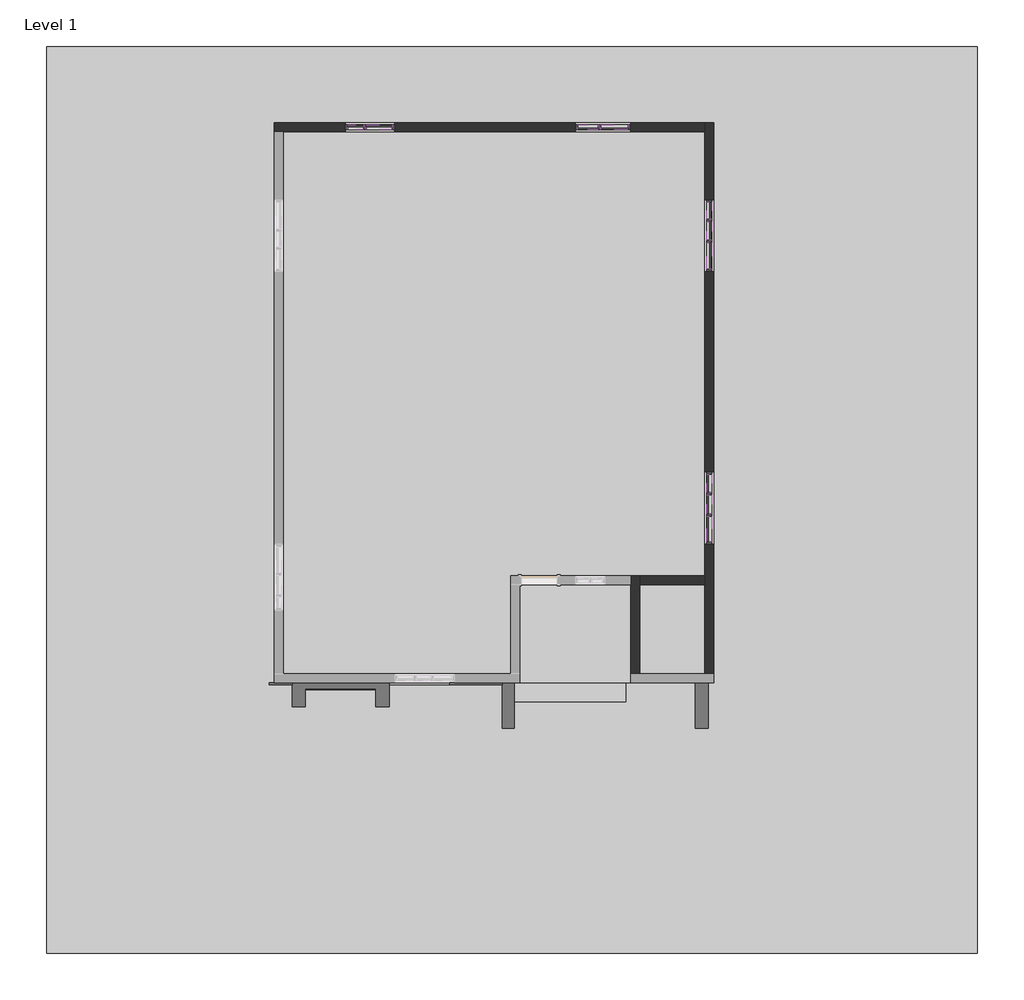
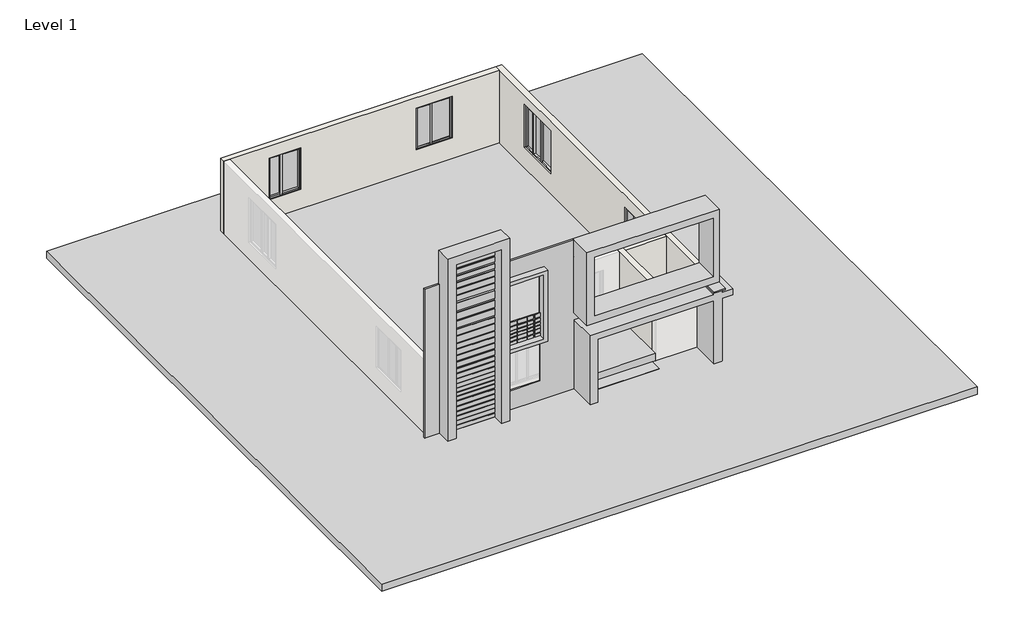
# One storey, part 2 of 2: 34 members, 10 plates, 4 walls, 2 proxies.
"""IFC4 building model written with IfcOpenShell, lengths in millimetres."""

from ifc_helpers import new_model, si_unit, origin, origin_with_axes, place, context, project, spatial, polyline, outline, extrude, faceted_brep, transform, mapped, element, save
from components import generic_models_1_generic_models_1_010c0d49, generic_models_2_generic_models_2_25274e54, member_dc106669, member_969ca954, member_86d06fe4, member_dad99500, member_5e920210, member_530c9cc4, member_2b79973d, member_c33c434a, member_337b6441, member_f67b4128, member_6fb4a552, member_0b7646a3, member_b956c4f6, member_d8304dce, member_273748f4, member_7c181f63, member_bc773a83, member_183d059d, system_panel_glazed_46d50955, system_panel_glazed_6f1fa804, system_panel_glazed_7e68e824, system_panel_glazed_aca50f87, system_panel_glazed_bef0ddaa, system_panel_glazed_29222c04, system_panel_glazed_73ac8250, system_panel_glazed_52b4f5c1, system_panel_glazed_3b3b315d, system_panel_glazed_762caeb2

model = new_model("IFC4")

# Units and contexts
model_context = context("Model", 3, world=origin())
ifc_project = project(units=[si_unit("LENGTHUNIT", "METRE", prefix="MILLI")], contexts=[model_context])

# Site, building, storey
site = spatial("IfcSite", under=ifc_project)
building = spatial("IfcBuilding", under=site)
storey = spatial("IfcBuildingStorey", under=building, Name="Level 1", Elevation=0.0)

# Proxies
placement = place(None, origin())
generic_models_1_generic_models_1_shape = generic_models_1_generic_models_1_010c0d49(model_context)
element("IfcBuildingElementProxy", 1, Name="Generic Models 1 : Generic Models 1", ObjectType="Generic Models 1 : Generic Models 1", at=placement, inside=storey, context=model_context, shape_type="MappedRepresentation", body=[
    mapped(generic_models_1_generic_models_1_shape, transform((0.0, 0.0, 0.0), x_axis=(1.0, 0.0, 0.0), y_axis=(0.0, 1.0, 0.0), z_axis=(0.0, 0.0, 1.0))),
])
generic_models_2_generic_models_2_shape = generic_models_2_generic_models_2_25274e54(model_context)
element("IfcBuildingElementProxy", 2, Name="Generic Models 2 : Generic Models 2", ObjectType="Generic Models 2 : Generic Models 2", at=placement, inside=storey, context=model_context, shape_type="MappedRepresentation", body=[
    mapped(generic_models_2_generic_models_2_shape, transform((-134.3868469, 0.0, -162.5364257), x_axis=(1.0, 0.0, 0.0), y_axis=(0.0, 1.0, 0.0), z_axis=(0.0, 0.0, 1.0))),
])

# Members
member_shape = member_dc106669(model_context)
element("IfcMember", 3, ObjectType="Rectangular Mullion : 2.5\" x 5\" rectangular", at=placement, inside=storey, context=model_context, shape_type="MappedRepresentation", body=[
    mapped(member_shape, transform((-14463.3781629, -790.0678064, 2550.7938638), x_axis=(0.0, 0.0, 1.0), y_axis=(0.0, -1.0, 0.0), z_axis=(1.0, 0.0, 0.0))),
])
element("IfcMember", 4, ObjectType="Rectangular Mullion : 2.5\" x 5\" rectangular", at=placement, inside=storey, context=model_context, shape_type="MappedRepresentation", body=[
    mapped(member_shape, transform((-14876.1281629, -790.0678064, 803.2813363), x_axis=(0.0, 0.0, -1.0), y_axis=(0.0, -1.0, 0.0), z_axis=(-1.0, 0.0, 0.0))),
])
member_2_shape = member_969ca954(model_context)
element("IfcMember", 5, ObjectType="Rectangular Mullion : 2.5\" x 5\" rectangular", at=placement, inside=storey, context=model_context, shape_type="MappedRepresentation", body=[
    mapped(member_2_shape, transform((-5719.4281629, -10029.3178064, 840.8595188), x_axis=(0.0, 0.0, -1.0), y_axis=(1.0, 0.0, 0.0), z_axis=(0.0, -1.0, 0.0))),
])
member_3_shape = member_86d06fe4(model_context)
element("IfcMember", 6, ObjectType="Rectangular Mullion : 2.5\" x 5\" rectangular", at=placement, inside=storey, context=model_context, shape_type="MappedRepresentation", body=[
    mapped(member_3_shape, transform((-5719.4281629, -10575.4178064, 840.8595188), x_axis=(0.0, 0.0, -1.0), y_axis=(1.0, 0.0, 0.0), z_axis=(0.0, -1.0, 0.0))),
])
member_4_shape = member_dad99500(model_context)
element("IfcMember", 7, ObjectType="Rectangular Mullion : 2.5\" x 5\" rectangular", at=placement, inside=storey, context=model_context, shape_type="MappedRepresentation", body=[
    mapped(member_4_shape, transform((-5719.4281629, -11280.2678064, 840.8595188), x_axis=(0.0, 0.0, -1.0), y_axis=(1.0, 0.0, 0.0), z_axis=(0.0, -1.0, 0.0))),
])
member_5_shape = member_5e920210(model_context)
element("IfcMember", 8, ObjectType="Rectangular Mullion : 2.5\" x 5\" rectangular", at=placement, inside=storey, context=model_context, shape_type="MappedRepresentation", body=[
    mapped(member_5_shape, transform((-5719.4281629, -10607.1678064, 840.8595188), x_axis=(0.0, 1.0, 0.0), y_axis=(1.0, 0.0, 0.0), z_axis=(0.0, 0.0, -1.0))),
])
element("IfcMember", 9, ObjectType="Rectangular Mullion : 2.5\" x 5\" rectangular", at=placement, inside=storey, context=model_context, shape_type="MappedRepresentation", body=[
    mapped(member_5_shape, transform((-5719.4281629, -10061.0678064, 840.8595188), x_axis=(0.0, 1.0, 0.0), y_axis=(1.0, 0.0, 0.0), z_axis=(0.0, 0.0, -1.0))),
])
element("IfcMember", 10, ObjectType="Rectangular Mullion : 2.5\" x 5\" rectangular", at=placement, inside=storey, context=model_context, shape_type="MappedRepresentation", body=[
    mapped(member_3_shape, transform((-5719.4281629, -10092.8178064, 2522.9339832), x_axis=(0.0, 0.0, 1.0), y_axis=(1.0, 0.0, 0.0), z_axis=(0.0, 1.0, 0.0))),
])
element("IfcMember", 11, ObjectType="Rectangular Mullion : 2.5\" x 5\" rectangular", at=placement, inside=storey, context=model_context, shape_type="MappedRepresentation", body=[
    mapped(member_4_shape, transform((-5719.4281629, -10638.9178064, 2522.9339832), x_axis=(0.0, 0.0, 1.0), y_axis=(1.0, 0.0, 0.0), z_axis=(0.0, 1.0, 0.0))),
])
element("IfcMember", 12, ObjectType="Rectangular Mullion : 2.5\" x 5\" rectangular", at=placement, inside=storey, context=model_context, shape_type="MappedRepresentation", body=[
    mapped(member_2_shape, transform((-5719.4281629, -9578.4678064, 2522.9339832), x_axis=(0.0, 0.0, 1.0), y_axis=(1.0, 0.0, 0.0), z_axis=(0.0, 1.0, 0.0))),
])
member_6_shape = member_530c9cc4(model_context)
element("IfcMember", 13, ObjectType="Rectangular Mullion : 2.5\" x 5\" rectangular", at=placement, inside=storey, context=model_context, shape_type="MappedRepresentation", body=[
    mapped(member_6_shape, transform((-5719.4281629, -9514.9678064, 840.8595188), x_axis=(0.0, 1.0, 0.0), y_axis=(1.0, 0.0, 0.0), z_axis=(0.0, 0.0, -1.0))),
])
element("IfcMember", 14, ObjectType="Rectangular Mullion : 2.5\" x 5\" rectangular", at=placement, inside=storey, context=model_context, shape_type="MappedRepresentation", body=[
    mapped(member_6_shape, transform((-5719.4281629, -11343.7678064, 2522.9339832), x_axis=(0.0, -1.0, 0.0), y_axis=(1.0, 0.0, 0.0), z_axis=(0.0, 0.0, 1.0))),
])
member_7_shape = member_2b79973d(model_context)
element("IfcMember", 15, ObjectType="Rectangular Mullion : 2.5\" x 5\" rectangular", at=placement, inside=storey, context=model_context, shape_type="MappedRepresentation", body=[
    mapped(member_7_shape, transform((-5719.4281629, -3653.9178064, 2661.4285089), x_axis=(0.0, 0.0, 1.0), y_axis=(-1.0, 0.0, 0.0), z_axis=(0.0, -1.0, 0.0))),
])
member_8_shape = member_c33c434a(model_context)
element("IfcMember", 16, ObjectType="Rectangular Mullion : 2.5\" x 5\" rectangular", at=placement, inside=storey, context=model_context, shape_type="MappedRepresentation", body=[
    mapped(member_8_shape, transform((-5719.4281629, -4384.1678064, 2661.4285089), x_axis=(0.0, 0.0, 1.0), y_axis=(-1.0, 0.0, 0.0), z_axis=(0.0, -1.0, 0.0))),
])
member_9_shape = member_337b6441(model_context)
element("IfcMember", 17, ObjectType="Rectangular Mullion : 2.5\" x 5\" rectangular", at=placement, inside=storey, context=model_context, shape_type="MappedRepresentation", body=[
    mapped(member_9_shape, transform((-5719.4281629, -3152.2678064, 856.0019171), x_axis=(0.0, -1.0, 0.0), y_axis=(-1.0, 0.0, 0.0), z_axis=(0.0, 0.0, -1.0))),
])
element("IfcMember", 18, ObjectType="Rectangular Mullion : 2.5\" x 5\" rectangular", at=placement, inside=storey, context=model_context, shape_type="MappedRepresentation", body=[
    mapped(member_9_shape, transform((-5719.4281629, -3685.6678064, 856.0019171), x_axis=(0.0, -1.0, 0.0), y_axis=(-1.0, 0.0, 0.0), z_axis=(0.0, 0.0, -1.0))),
])
element("IfcMember", 19, ObjectType="Rectangular Mullion : 2.5\" x 5\" rectangular", at=placement, inside=storey, context=model_context, shape_type="MappedRepresentation", body=[
    mapped(member_7_shape, transform((-5719.4281629, -3184.0178064, 856.0019171), x_axis=(0.0, 0.0, -1.0), y_axis=(-1.0, 0.0, 0.0), z_axis=(0.0, 1.0, 0.0))),
])
element("IfcMember", 20, ObjectType="Rectangular Mullion : 2.5\" x 5\" rectangular", at=placement, inside=storey, context=model_context, shape_type="MappedRepresentation", body=[
    mapped(member_8_shape, transform((-5719.4281629, -3717.4178064, 856.0019171), x_axis=(0.0, 0.0, -1.0), y_axis=(-1.0, 0.0, 0.0), z_axis=(0.0, 1.0, 0.0))),
])
member_10_shape = member_f67b4128(model_context)
element("IfcMember", 21, ObjectType="Rectangular Mullion : 2.5\" x 5\" rectangular", at=placement, inside=storey, context=model_context, shape_type="MappedRepresentation", body=[
    mapped(member_10_shape, transform((-5719.4281629, -4447.6678064, 856.0019171), x_axis=(0.0, -1.0, 0.0), y_axis=(-1.0, 0.0, 0.0), z_axis=(0.0, 0.0, -1.0))),
])
member_11_shape = member_6fb4a552(model_context)
element("IfcMember", 22, ObjectType="Rectangular Mullion : 2.5\" x 5\" rectangular", at=placement, inside=storey, context=model_context, shape_type="MappedRepresentation", body=[
    mapped(member_11_shape, transform((-5719.4281629, -3120.5178064, 2661.4285089), x_axis=(0.0, 0.0, 1.0), y_axis=(-1.0, 0.0, 0.0), z_axis=(0.0, -1.0, 0.0))),
])
element("IfcMember", 23, ObjectType="Rectangular Mullion : 2.5\" x 5\" rectangular", at=placement, inside=storey, context=model_context, shape_type="MappedRepresentation", body=[
    mapped(member_11_shape, transform((-5719.4281629, -2682.3678064, 856.0019171), x_axis=(0.0, 0.0, -1.0), y_axis=(-1.0, 0.0, 0.0), z_axis=(0.0, 1.0, 0.0))),
])
element("IfcMember", 24, ObjectType="Rectangular Mullion : 2.5\" x 5\" rectangular", at=placement, inside=storey, context=model_context, shape_type="MappedRepresentation", body=[
    mapped(member_10_shape, transform((-5719.4281629, -2618.8678064, 2661.4285089), x_axis=(0.0, 1.0, 0.0), y_axis=(-1.0, 0.0, 0.0), z_axis=(0.0, 0.0, 1.0))),
])
member_12_shape = member_0b7646a3(model_context)
element("IfcMember", 25, ObjectType="Rectangular Mullion : 2.5\" x 5\" rectangular", at=placement, inside=storey, context=model_context, shape_type="MappedRepresentation", body=[
    mapped(member_12_shape, transform((-9046.8281629, -790.0678064, 2606.6947773), x_axis=(0.0, 0.0, 1.0), y_axis=(0.0, 1.0, 0.0), z_axis=(-1.0, 0.0, 0.0))),
])
member_13_shape = member_b956c4f6(model_context)
element("IfcMember", 26, ObjectType="Rectangular Mullion : 2.5\" x 5\" rectangular", at=placement, inside=storey, context=model_context, shape_type="MappedRepresentation", body=[
    mapped(member_13_shape, transform((-8468.9781629, -790.0678064, 2606.6947773), x_axis=(0.0, 0.0, 1.0), y_axis=(0.0, 1.0, 0.0), z_axis=(-1.0, 0.0, 0.0))),
])
member_14_shape = member_d8304dce(model_context)
element("IfcMember", 27, ObjectType="Rectangular Mullion : 2.5\" x 5\" rectangular", at=placement, inside=storey, context=model_context, shape_type="MappedRepresentation", body=[
    mapped(member_14_shape, transform((-8500.7281629, -790.0678064, 862.6148637), x_axis=(-1.0, 0.0, 0.0), y_axis=(0.0, 1.0, 0.0), z_axis=(0.0, 0.0, -1.0))),
])
element("IfcMember", 28, ObjectType="Rectangular Mullion : 2.5\" x 5\" rectangular", at=placement, inside=storey, context=model_context, shape_type="MappedRepresentation", body=[
    mapped(member_12_shape, transform((-8532.4781629, -790.0678064, 862.6148637), x_axis=(0.0, 0.0, -1.0), y_axis=(0.0, 1.0, 0.0), z_axis=(1.0, 0.0, 0.0))),
])
element("IfcMember", 29, ObjectType="Rectangular Mullion : 2.5\" x 5\" rectangular", at=placement, inside=storey, context=model_context, shape_type="MappedRepresentation", body=[
    mapped(member_13_shape, transform((-7764.1281629, -790.0678064, 862.6148637), x_axis=(0.0, 0.0, -1.0), y_axis=(0.0, 1.0, 0.0), z_axis=(1.0, 0.0, 0.0))),
])
member_15_shape = member_273748f4(model_context)
element("IfcMember", 30, ObjectType="Rectangular Mullion : 2.5\" x 5\" rectangular", at=placement, inside=storey, context=model_context, shape_type="MappedRepresentation", body=[
    mapped(member_15_shape, transform((-9110.3281629, -790.0678064, 862.6148637), x_axis=(-1.0, 0.0, 0.0), y_axis=(0.0, 1.0, 0.0), z_axis=(0.0, 0.0, -1.0))),
])
element("IfcMember", 31, ObjectType="Rectangular Mullion : 2.5\" x 5\" rectangular", at=placement, inside=storey, context=model_context, shape_type="MappedRepresentation", body=[
    mapped(member_15_shape, transform((-7700.6281629, -790.0678064, 2606.6947773), x_axis=(1.0, 0.0, 0.0), y_axis=(0.0, 1.0, 0.0), z_axis=(0.0, 0.0, 1.0))),
])
member_16_shape = member_7c181f63(model_context)
element("IfcMember", 32, ObjectType="Rectangular Mullion : 2.5\" x 5\" rectangular", at=placement, inside=storey, context=model_context, shape_type="MappedRepresentation", body=[
    mapped(member_16_shape, transform((-13745.8281629, -790.0678064, 2550.7938638), x_axis=(0.0, 0.0, 1.0), y_axis=(0.0, -1.0, 0.0), z_axis=(1.0, 0.0, 0.0))),
])
member_17_shape = member_bc773a83(model_context)
element("IfcMember", 33, ObjectType="Rectangular Mullion : 2.5\" x 5\" rectangular", at=placement, inside=storey, context=model_context, shape_type="MappedRepresentation", body=[
    mapped(member_17_shape, transform((-14431.6281629, -790.0678064, 803.2813363), x_axis=(1.0, 0.0, 0.0), y_axis=(0.0, -1.0, 0.0), z_axis=(0.0, 0.0, -1.0))),
])
element("IfcMember", 34, ObjectType="Rectangular Mullion : 2.5\" x 5\" rectangular", at=placement, inside=storey, context=model_context, shape_type="MappedRepresentation", body=[
    mapped(member_16_shape, transform((-14399.8781629, -790.0678064, 803.2813363), x_axis=(0.0, 0.0, -1.0), y_axis=(0.0, -1.0, 0.0), z_axis=(-1.0, 0.0, 0.0))),
])
member_18_shape = member_183d059d(model_context)
element("IfcMember", 35, ObjectType="Rectangular Mullion : 2.5\" x 5\" rectangular", at=placement, inside=storey, context=model_context, shape_type="MappedRepresentation", body=[
    mapped(member_18_shape, transform((-14939.6281629, -790.0678064, 2550.7938638), x_axis=(-1.0, 0.0, 0.0), y_axis=(0.0, -1.0, 0.0), z_axis=(0.0, 0.0, 1.0))),
])
element("IfcMember", 36, ObjectType="Rectangular Mullion : 2.5\" x 5\" rectangular", at=placement, inside=storey, context=model_context, shape_type="MappedRepresentation", body=[
    mapped(member_18_shape, transform((-13682.3281629, -790.0678064, 803.2813363), x_axis=(1.0, 0.0, 0.0), y_axis=(0.0, -1.0, 0.0), z_axis=(0.0, 0.0, -1.0))),
])

# Plates
system_panel_glazed_shape = system_panel_glazed_46d50955(model_context)
element("IfcPlate", 37, ObjectType="System Panel : Glazed", at=placement, inside=storey, context=model_context, shape_type="MappedRepresentation", body=[
    mapped(system_panel_glazed_shape, transform((-5719.4281629, -10959.5928064, 904.3595188), x_axis=(0.0, 1.0, 0.0), y_axis=(-1.0, 0.0, 0.0), z_axis=(0.0, 0.0, 1.0))),
])
system_panel_glazed_2_shape = system_panel_glazed_6f1fa804(model_context)
element("IfcPlate", 38, ObjectType="System Panel : Glazed", at=placement, inside=storey, context=model_context, shape_type="MappedRepresentation", body=[
    mapped(system_panel_glazed_2_shape, transform((-5719.4281629, -10334.1178064, 904.3595188), x_axis=(0.0, 1.0, 0.0), y_axis=(-1.0, 0.0, 0.0), z_axis=(0.0, 0.0, 1.0))),
])
system_panel_glazed_3_shape = system_panel_glazed_7e68e824(model_context)
element("IfcPlate", 39, ObjectType="System Panel : Glazed", at=placement, inside=storey, context=model_context, shape_type="MappedRepresentation", body=[
    mapped(system_panel_glazed_3_shape, transform((-5719.4281629, -9803.8928064, 904.3595188), x_axis=(0.0, 1.0, 0.0), y_axis=(-1.0, 0.0, 0.0), z_axis=(0.0, 0.0, 1.0))),
])
system_panel_glazed_4_shape = system_panel_glazed_aca50f87(model_context)
element("IfcPlate", 40, ObjectType="System Panel : Glazed", at=placement, inside=storey, context=model_context, shape_type="MappedRepresentation", body=[
    mapped(system_panel_glazed_4_shape, transform((-5719.4281629, -4050.7928064, 919.5019171), x_axis=(0.0, -1.0, 0.0), y_axis=(1.0, 0.0, 0.0), z_axis=(0.0, 0.0, 1.0))),
])
system_panel_glazed_5_shape = system_panel_glazed_bef0ddaa(model_context)
element("IfcPlate", 41, ObjectType="System Panel : Glazed", at=placement, inside=storey, context=model_context, shape_type="MappedRepresentation", body=[
    mapped(system_panel_glazed_5_shape, transform((-5719.4281629, -3418.9678064, 919.5019171), x_axis=(0.0, -1.0, 0.0), y_axis=(1.0, 0.0, 0.0), z_axis=(0.0, 0.0, 1.0))),
])
system_panel_glazed_6_shape = system_panel_glazed_29222c04(model_context)
element("IfcPlate", 42, ObjectType="System Panel : Glazed", at=placement, inside=storey, context=model_context, shape_type="MappedRepresentation", body=[
    mapped(system_panel_glazed_6_shape, transform((-5719.4281629, -2901.4428064, 919.5019171), x_axis=(0.0, -1.0, 0.0), y_axis=(1.0, 0.0, 0.0), z_axis=(0.0, 0.0, 1.0))),
])
system_panel_glazed_7_shape = system_panel_glazed_73ac8250(model_context)
element("IfcPlate", 43, ObjectType="System Panel : Glazed", at=placement, inside=storey, context=model_context, shape_type="MappedRepresentation", body=[
    mapped(system_panel_glazed_7_shape, transform((-8116.5531629, -790.0678064, 926.1148637), x_axis=(-1.0, 0.0, 0.0), y_axis=(0.0, -1.0, 0.0), z_axis=(0.0, 0.0, 1.0))),
])
system_panel_glazed_8_shape = system_panel_glazed_52b4f5c1(model_context)
element("IfcPlate", 44, ObjectType="System Panel : Glazed", at=placement, inside=storey, context=model_context, shape_type="MappedRepresentation", body=[
    mapped(system_panel_glazed_8_shape, transform((-8789.6531629, -790.0678064, 926.1148637), x_axis=(-1.0, 0.0, 0.0), y_axis=(0.0, -1.0, 0.0), z_axis=(0.0, 0.0, 1.0))),
])
system_panel_glazed_9_shape = system_panel_glazed_3b3b315d(model_context)
element("IfcPlate", 45, ObjectType="System Panel : Glazed", at=placement, inside=storey, context=model_context, shape_type="MappedRepresentation", body=[
    mapped(system_panel_glazed_9_shape, transform((-14669.7531629, -790.0678064, 866.7813363), x_axis=(1.0, 0.0, 0.0), y_axis=(0.0, 1.0, 0.0), z_axis=(0.0, 0.0, 1.0))),
])
system_panel_glazed_10_shape = system_panel_glazed_762caeb2(model_context)
element("IfcPlate", 46, ObjectType="System Panel : Glazed", at=placement, inside=storey, context=model_context, shape_type="MappedRepresentation", body=[
    mapped(system_panel_glazed_10_shape, transform((-14072.8531629, -790.0678064, 866.7813363), x_axis=(1.0, 0.0, 0.0), y_axis=(0.0, 1.0, 0.0), z_axis=(0.0, 0.0, 1.0))),
])

# Walls
element("IfcWall", 47, ObjectType="9\"", at=placement, inside=storey, context=model_context, shape_type="Brep", body=[
    faceted_brep([(-5605.1281629, -14620.3678064, 0.0), (-5605.1281629, -675.7678064, 0.0), (-5605.1281629, -675.7678064, 3048.0), (-5605.1281629, -14620.3678064, 3048.0), (-5605.1281629, -11343.7678064, 840.8595188), (-5605.1281629, -11343.7678064, 2522.9339832), (-5605.1281629, -9514.9678064, 2522.9339832), (-5605.1281629, -9514.9678064, 840.8595188), (-5605.1281629, -2618.8678064, 2661.4285089), (-5605.1281629, -2618.8678064, 856.0019171), (-5605.1281629, -4447.6678064, 856.0019171), (-5605.1281629, -4447.6678064, 2661.4285089), (-5833.7281629, -675.7678064, 0.0), (-5833.7281629, -904.3678064, 0.0), (-5833.7281629, -12143.8678064, 0.0), (-5833.7281629, -12372.4678064, 0.0), (-5833.7281629, -14620.3678064, 0.0), (-5833.7281629, -14620.3678064, 3048.0), (-5833.7281629, -12372.4678064, 3048.0), (-5833.7281629, -12143.8678064, 3048.0), (-5833.7281629, -904.3678064, 3048.0), (-5833.7281629, -675.7678064, 3048.0), (-5833.7281629, -11343.7678064, 2522.9339832), (-5833.7281629, -11343.7678064, 840.8595188), (-5833.7281629, -9514.9678064, 840.8595188), (-5833.7281629, -9514.9678064, 2522.9339832), (-5833.7281629, -2618.8678064, 856.0019171), (-5833.7281629, -2618.8678064, 2661.4285089), (-5833.7281629, -4447.6678064, 2661.4285089), (-5833.7281629, -4447.6678064, 856.0019171)], [[[0, 1, 2, 3], [4, 5, 6, 7], [8, 9, 10, 11]], [[12, 13, 14, 15, 16, 17, 18, 19, 20, 21], [22, 23, 24, 25], [26, 27, 28, 29]], [[1, 0, 16, 15, 14, 13, 12]], [[3, 2, 21, 20, 19, 18, 17]], [[0, 3, 17, 16]], [[2, 1, 12, 21]], [[4, 23, 22, 5]], [[5, 22, 25, 6]], [[6, 25, 24, 7]], [[23, 4, 7, 24]], [[26, 9, 8, 27]], [[27, 8, 11, 28]], [[10, 29, 28, 11]], [[9, 26, 29, 10]]]),
])
element("IfcWall", 48, ObjectType="9\"", at=placement, inside=storey, context=model_context, shape_type="Brep", body=[
    faceted_brep([(-5833.7281629, -675.7678064, 0.0), (-16730.3281629, -675.7678064, 0.0), (-16730.3281629, -675.7678064, 3048.0), (-5833.7281629, -675.7678064, 3048.0), (-7700.6281629, -675.7678064, 862.6148637), (-7700.6281629, -675.7678064, 2606.6947773), (-9110.3281629, -675.7678064, 2606.6947773), (-9110.3281629, -675.7678064, 862.6148637), (-14939.6281629, -675.7678064, 2550.7938638), (-14939.6281629, -675.7678064, 803.2813363), (-13682.3281629, -675.7678064, 803.2813363), (-13682.3281629, -675.7678064, 2550.7938638), (-16730.3281629, -904.3678064, 0.0), (-16501.7281629, -904.3678064, 0.0), (-5833.7281629, -904.3678064, 0.0), (-5833.7281629, -904.3678064, 3048.0), (-16501.7281629, -904.3678064, 3048.0), (-16730.3281629, -904.3678064, 3048.0), (-7700.6281629, -904.3678064, 2606.6947773), (-7700.6281629, -904.3678064, 862.6148637), (-9110.3281629, -904.3678064, 862.6148637), (-9110.3281629, -904.3678064, 2606.6947773), (-14939.6281629, -904.3678064, 803.2813363), (-14939.6281629, -904.3678064, 2550.7938638), (-13682.3281629, -904.3678064, 2550.7938638), (-13682.3281629, -904.3678064, 803.2813363)], [[[0, 1, 2, 3], [4, 5, 6, 7], [8, 9, 10, 11]], [[12, 13, 14, 15, 16, 17], [18, 19, 20, 21], [22, 23, 24, 25]], [[1, 0, 14, 13, 12]], [[3, 2, 17, 16, 15]], [[0, 3, 15, 14]], [[2, 1, 12, 17]], [[4, 19, 18, 5]], [[5, 18, 21, 6]], [[6, 21, 20, 7]], [[19, 4, 7, 20]], [[22, 9, 8, 23]], [[23, 8, 11, 24]], [[10, 25, 24, 11]], [[9, 22, 25, 10]]]),
])
element("IfcWall", 49, ObjectType="9\"", at=placement, inside=storey, context=model_context, shape_type="Brep", body=[
    faceted_brep([(-7472.0281629, -14620.3678064, 0.0), (-7472.0281629, -12372.4678064, 0.0), (-7472.0281629, -12143.8678064, 0.0), (-7472.0281629, -12143.8678064, 3048.0), (-7472.0281629, -12372.4678064, 3048.0), (-7472.0281629, -14620.3678064, 3048.0), (-7700.6281629, -14620.3678064, 0.0), (-7700.6281629, -14620.3678064, 3048.0), (-7700.6281629, -12372.4678064, 3048.0), (-7700.6281629, -12143.8678064, 3048.0), (-7700.6281629, -12143.8678064, 0.0), (-7700.6281629, -12372.4678064, 0.0)], [[[0, 1, 2, 3, 4, 5]], [[6, 7, 8, 9, 10, 11]], [[2, 1, 0, 6, 11, 10]], [[5, 4, 3, 9, 8, 7]], [[0, 5, 7, 6]], [[3, 2, 10, 9]]]),
])
element("IfcWall", 50, ObjectType="9\"", at=placement, inside=storey, context=model_context, shape_type="SweptSolid", body=[
    extrude(outline(polyline([(-5833.7281629, -12372.4678064), (-7472.0281629, -12372.4678064), (-7472.0281629, -12143.8678064), (-5833.7281629, -12143.8678064), (-5833.7281629, -12372.4678064)])), origin_with_axes(), (0.0, 0.0, 1.0), 3048.0),
])

save(model, "model.ifc")

# Revit data of these elements
# Type "Rectangular Mullion : 2.5\" x 5\" rectangular"
#   built-in parameter 1007304 = 0.416667 (stored number, unit not read)
#   built-in parameter 1007301 = 0.104167 (stored number, unit not read)
#   built-in parameter 1007300 = 0.104167 (stored number, unit not read)
# Type "System Panel : Glazed"
#   Construction Type Id = "GSP4R"
#   Analytic Construction = "1/8 in Pilkington single glazing"
#   Visual Light Transmittance = 0.9
#   Solar Heat Gain Coefficient = 0.86
#   Heat Transfer Coefficient (U) = 1.18115 BTU/(h·ft²·°F)
#   Define Thermal Properties by = 1
# Type "9\""
#   Assembly Code = "B2010"
#   Layers, outside or top first: 0' - 9" no material (function 1)
# Element 1 (IfcBuildingElementProxy, "Generic Models 1 : Generic Models 1")
#   Phase Created = New Construction
# Element 2 (IfcBuildingElementProxy, "Generic Models 2 : Generic Models 2")
#   Phase Created = New Construction
# Elements 3, 4, 5, 6, 7, 8, 9, 10, 11, 12, 13, 14, 15, 16, 17, 18, 19, 20, 21, 22, 23, 24, 25, 26, 27, 28, 29, 30, 31, 32, 33, 34, 35, 36 (IfcMember, "Rectangular Mullion : 2.5\" x 5\" rectangular")
#   Phase Created = New Construction
#   Materials on its faces: "Aluminum"
# Elements 37, 38, 39, 40, 41, 42, 43, 44, 45, 46 (IfcPlate, "System Panel : Glazed")
#   Phase Created = New Construction
#   Materials on its faces: "Glass"
# Elements 47, 48, 49, 50 (IfcWall, "9\"")
#   Top Offset = 0' - 0"
#   Base Offset = 0' - 0"
#   Unconnected Height = 10' - 0"
#   wall height = 10' - 0"
#   Phase Created = New Construction
#   Base Constraint = Level 1
#   Materials on its faces: "Default Wall"
# Materials
#   "Aluminum": class "Metal", colour RGB 247 247 247, transparency 0, Description = "Aluminum 6061", Cost = 0
#   "Glass": class "Glass", colour RGB 0 128 192, transparency 0.75, Description = "Soda Lime Glass", Cost = 0
#   "Default Wall": colour RGB 128 128 128, transparency 0, Cost = 0
